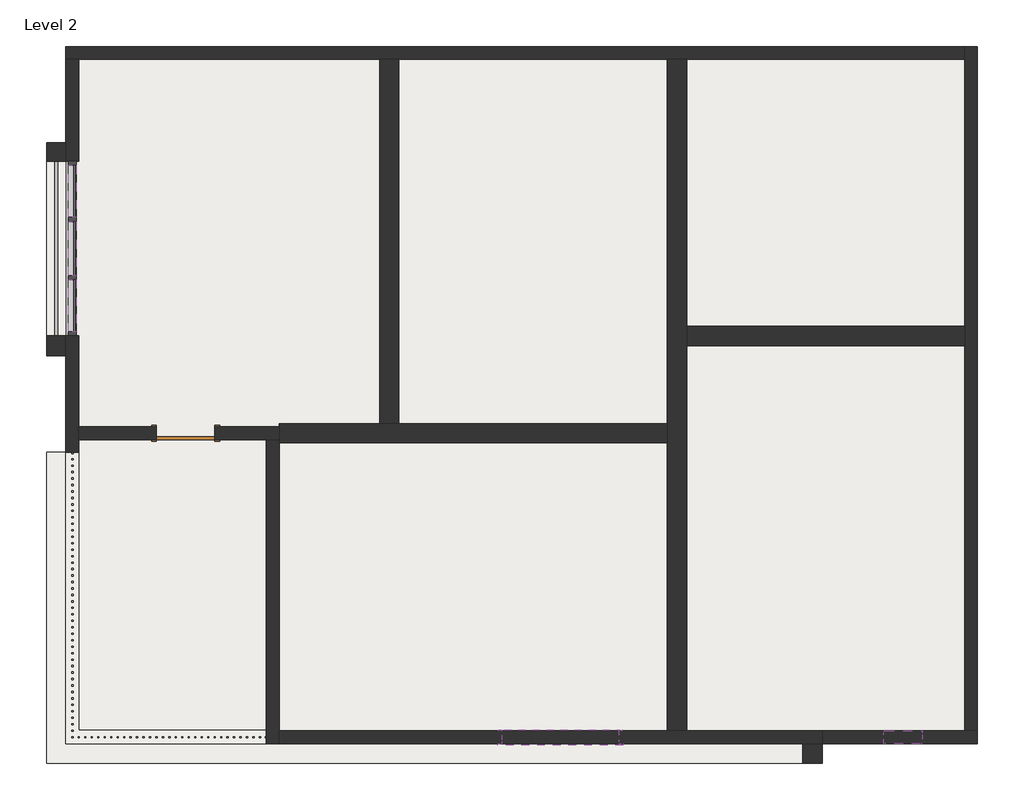
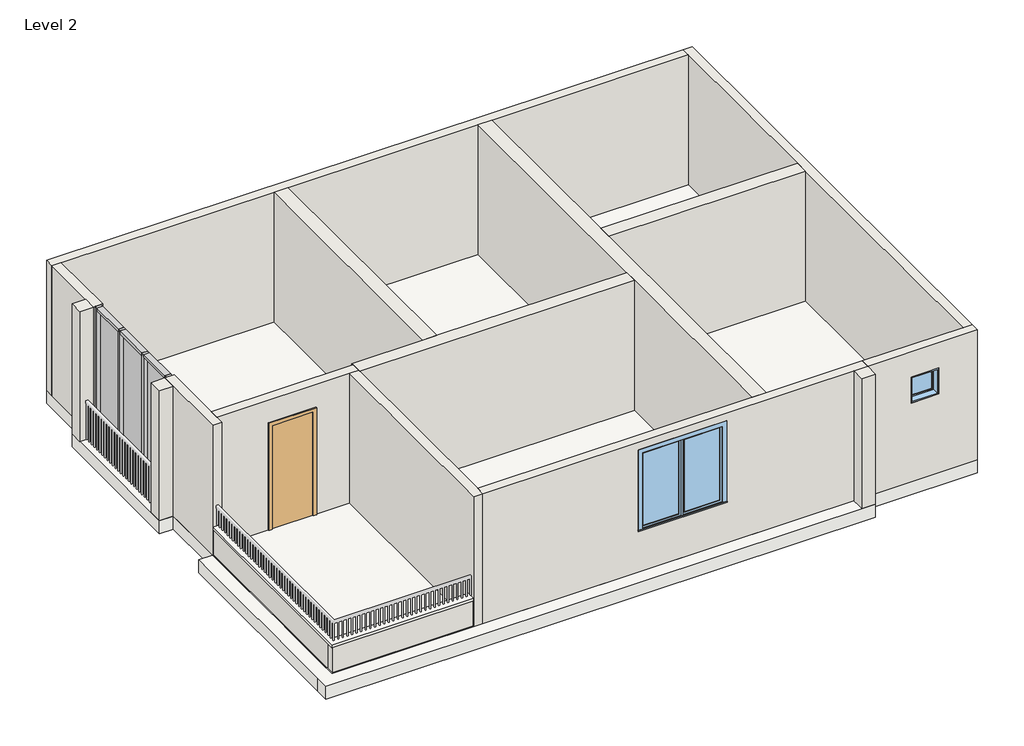
# One storey, part 1 of 2: 17 walls, 10 members, 3 plates, 3 slabs, 2 windows, 1 door.
"""IFC4 building model written with IfcOpenShell, lengths in millimetres."""

from ifc_helpers import new_model, si_unit, frame, origin, place, context, project, spatial, polyline, outline, extrude, faceted_brep, transform, mapped, element, save
from components import door_f936a269, member_eaba9652, member_3f395ae9, member_c17f1be2, member_d2e7e466, system_panel_glazed_52d31088, system_panel_glazed_f0722de2, window_97c6202a, window_6846e476

model = new_model("IFC4")

# Units and contexts
model_context = context("Model", 3, world=origin())
ifc_project = project(units=[si_unit("LENGTHUNIT", "METRE", prefix="MILLI")], contexts=[model_context])

# Site, building, storey
site = spatial("IfcSite", under=ifc_project)
building = spatial("IfcBuilding", under=site)
storey = spatial("IfcBuildingStorey", under=building, Name="Level 2", Elevation=3048.0)

# Door
placement = place(None, origin())
door_shape = door_f936a269(model_context)
element("IfcDoor", 1, ObjectType="Single-Flush : 36\" x 96\"", at=placement, inside=storey, context=model_context, shape_type="MappedRepresentation", body=[
    mapped(door_shape, transform((-16449.2169582, -4610.4617616, 3352.8), x_axis=(-1.0, 0.0, 0.0), y_axis=(0.0, -1.0, 0.0), z_axis=(0.0, 0.0, 1.0))),
])

# Members
member_shape = member_eaba9652(model_context)
element("IfcMember", 2, ObjectType="Rectangular Mullion : 2.5\" x 5\" rectangular", at=placement, inside=storey, context=model_context, shape_type="MappedRepresentation", body=[
    mapped(member_shape, transform((-18227.2169582, -1251.3117616, 3352.8), x_axis=(0.0, -1.0, 0.0), y_axis=(-1.0, 0.0, 0.0), z_axis=(0.0, 0.0, -1.0))),
])
element("IfcMember", 3, ObjectType="Rectangular Mullion : 2.5\" x 5\" rectangular", at=placement, inside=storey, context=model_context, shape_type="MappedRepresentation", body=[
    mapped(member_shape, transform((-18227.2169582, -2165.7117616, 3352.8), x_axis=(0.0, -1.0, 0.0), y_axis=(-1.0, 0.0, 0.0), z_axis=(0.0, 0.0, -1.0))),
])
member_2_shape = member_3f395ae9(model_context)
element("IfcMember", 4, ObjectType="Rectangular Mullion : 2.5\" x 5\" rectangular", at=placement, inside=storey, context=model_context, shape_type="MappedRepresentation", body=[
    mapped(member_2_shape, transform((-18227.2169582, -3080.1117616, 3352.8), x_axis=(0.0, -1.0, 0.0), y_axis=(-1.0, 0.0, 0.0), z_axis=(0.0, 0.0, -1.0))),
])
element("IfcMember", 5, ObjectType="Rectangular Mullion : 2.5\" x 5\" rectangular", at=placement, inside=storey, context=model_context, shape_type="MappedRepresentation", body=[
    mapped(member_2_shape, transform((-18227.2169582, -336.9117616, 6400.8), x_axis=(0.0, 1.0, 0.0), y_axis=(-1.0, 0.0, 0.0), z_axis=(0.0, 0.0, 1.0))),
])
member_3_shape = member_c17f1be2(model_context)
element("IfcMember", 6, ObjectType="Rectangular Mullion : 2.5\" x 5\" rectangular", at=placement, inside=storey, context=model_context, shape_type="MappedRepresentation", body=[
    mapped(member_3_shape, transform((-18227.2169582, -3016.6117616, 6400.8), x_axis=(0.0, 0.0, 1.0), y_axis=(-1.0, 0.0, 0.0), z_axis=(0.0, -1.0, 0.0))),
])
element("IfcMember", 7, ObjectType="Rectangular Mullion : 2.5\" x 5\" rectangular", at=placement, inside=storey, context=model_context, shape_type="MappedRepresentation", body=[
    mapped(member_3_shape, transform((-18227.2169582, -1219.5617616, 6400.8), x_axis=(0.0, 0.0, 1.0), y_axis=(-1.0, 0.0, 0.0), z_axis=(0.0, -1.0, 0.0))),
])
element("IfcMember", 8, ObjectType="Rectangular Mullion : 2.5\" x 5\" rectangular", at=placement, inside=storey, context=model_context, shape_type="MappedRepresentation", body=[
    mapped(member_3_shape, transform((-18227.2169582, -400.4117616, 3352.8), x_axis=(0.0, 0.0, -1.0), y_axis=(-1.0, 0.0, 0.0), z_axis=(0.0, 1.0, 0.0))),
])
element("IfcMember", 9, ObjectType="Rectangular Mullion : 2.5\" x 5\" rectangular", at=placement, inside=storey, context=model_context, shape_type="MappedRepresentation", body=[
    mapped(member_3_shape, transform((-18227.2169582, -2197.4617616, 3352.8), x_axis=(0.0, 0.0, -1.0), y_axis=(-1.0, 0.0, 0.0), z_axis=(0.0, 1.0, 0.0))),
])
member_4_shape = member_d2e7e466(model_context)
element("IfcMember", 10, ObjectType="Rectangular Mullion : 2.5\" x 5\" rectangular", at=placement, inside=storey, context=model_context, shape_type="MappedRepresentation", body=[
    mapped(member_4_shape, transform((-18227.2169582, -1283.0617616, 3352.8), x_axis=(0.0, 0.0, -1.0), y_axis=(-1.0, 0.0, 0.0), z_axis=(0.0, 1.0, 0.0))),
])
element("IfcMember", 11, ObjectType="Rectangular Mullion : 2.5\" x 5\" rectangular", at=placement, inside=storey, context=model_context, shape_type="MappedRepresentation", body=[
    mapped(member_4_shape, transform((-18227.2169582, -2133.9617616, 6400.8), x_axis=(0.0, 0.0, 1.0), y_axis=(-1.0, 0.0, 0.0), z_axis=(0.0, -1.0, 0.0))),
])

# Plates
system_panel_glazed_shape = system_panel_glazed_52d31088(model_context)
element("IfcPlate", 12, ObjectType="System Panel : Glazed", at=placement, inside=storey, context=model_context, shape_type="MappedRepresentation", body=[
    mapped(system_panel_glazed_shape, transform((-18227.2169582, -809.9867616, 3416.3), x_axis=(0.0, -1.0, 0.0), y_axis=(1.0, 0.0, 0.0), z_axis=(0.0, 0.0, 1.0))),
])
element("IfcPlate", 13, ObjectType="System Panel : Glazed", at=placement, inside=storey, context=model_context, shape_type="MappedRepresentation", body=[
    mapped(system_panel_glazed_shape, transform((-18227.2169582, -2607.0367616, 3416.3), x_axis=(0.0, -1.0, 0.0), y_axis=(1.0, 0.0, 0.0), z_axis=(0.0, 0.0, 1.0))),
])
system_panel_glazed_2_shape = system_panel_glazed_f0722de2(model_context)
element("IfcPlate", 14, ObjectType="System Panel : Glazed", at=placement, inside=storey, context=model_context, shape_type="MappedRepresentation", body=[
    mapped(system_panel_glazed_2_shape, transform((-18227.2169582, -1708.5117616, 3416.3), x_axis=(0.0, -1.0, 0.0), y_axis=(1.0, 0.0, 0.0), z_axis=(0.0, 0.0, 1.0))),
])

# Slabs
element("IfcSlab", 15, ObjectType="Generic - 12\"", at=placement, inside=storey, context=model_context, shape_type="SweptSolid", body=[
    extrude(outline(polyline([(-18633.6169582, -41.6299243), (-18328.8169582, -41.6299243), (-18328.8169582, -3394.4299243), (-18633.6169582, -3394.4299243), (-18633.6169582, -41.6299243)])), frame((0.0, 0.0, 3048.0), z_axis=(0.0, 0.0, 1.0), x_axis=(1.0, 0.0, 0.0)), (0.0, 0.0, 1.0), 304.8),
    extrude(outline(polyline([(-18633.6169582, -4908.9117616), (-18328.8169582, -4908.9117616), (-18328.8169582, -9487.2617616), (-6444.7919582, -9487.2617616), (-6444.7919582, -9792.0617616), (-18633.6169582, -9792.0617616), (-18633.6169582, -9487.2617616), (-18633.6169582, -4908.9117616)])), frame((0.0, 0.0, 3048.0), z_axis=(0.0, 0.0, 1.0), x_axis=(1.0, 0.0, 0.0)), (0.0, 0.0, 1.0), 304.8),
])
element("IfcSlab", 16, ObjectType="Generic - 12\" 2", at=placement, inside=storey, context=model_context, shape_type="SweptSolid", body=[
    extrude(outline(polyline([(-4006.3919582, 1466.4882384), (-4006.3919582, -9487.2617616), (-18328.8169582, -9487.2617616), (-18328.8169582, 1466.4882384), (-4006.3919582, 1466.4882384)])), frame((0.0, 0.0, 3048.0), z_axis=(0.0, 0.0, 1.0), x_axis=(1.0, 0.0, 0.0)), (0.0, 0.0, 1.0), 304.8),
])
element("IfcSlab", 17, ObjectType="Generic - 2\"", at=placement, inside=storey, context=model_context, shape_type="SweptSolid", body=[
    extrude(outline(polyline([(-15179.2169582, -9487.2617616), (-18328.8169582, -9487.2617616), (-18328.8169582, -4908.9117616), (-18125.6169582, -4908.9117616), (-18125.6169582, -9277.7117616), (-15179.2169582, -9277.7117616), (-15179.2169582, -9309.4617616), (-15179.2169582, -9487.2617616)])), frame((0.0, 0.0, 3962.4), z_axis=(0.0, 0.0, 1.0), x_axis=(1.0, 0.0, 0.0)), (0.0, 0.0, 1.0), 50.8),
])

# Walls
element("IfcWall", 18, ObjectType="Generic - 12\" white", at=placement, inside=storey, context=model_context, shape_type="SweptSolid", body=[
    extrude(outline(polyline([(-18633.6169582, -336.9117616), (-18633.6169582, -41.6299243), (-18328.8169582, -41.6299243), (-18328.8169582, -336.9117616), (-18633.6169582, -336.9117616)])), frame((0.0, 0.0, 3352.8), z_axis=(0.0, 0.0, 1.0), x_axis=(1.0, 0.0, 0.0)), (0.0, 0.0, 1.0), 3048.0),
])
element("IfcWall", 19, ObjectType="Generic - 12\" white", at=placement, inside=storey, context=model_context, shape_type="SweptSolid", body=[
    extrude(outline(polyline([(-18328.8169582, -3080.1117616), (-18328.8169582, -3394.4299243), (-18633.6169582, -3394.4299243), (-18633.6169582, -3080.1117616), (-18328.8169582, -3080.1117616)])), frame((0.0, 0.0, 3352.8), z_axis=(0.0, 0.0, 1.0), x_axis=(1.0, 0.0, 0.0)), (0.0, 0.0, 1.0), 3048.0),
])
element("IfcWall", 20, ObjectType="Generic - 12\" white", at=placement, inside=storey, context=model_context, shape_type="SweptSolid", body=[
    extrude(outline(polyline([(-6749.5919582, -9487.2617616), (-6444.7919582, -9487.2617616), (-6444.7919582, -9792.0617616), (-6749.5919582, -9792.0617616), (-6749.5919582, -9487.2617616)])), frame((0.0, 0.0, 3352.8), z_axis=(0.0, 0.0, 1.0), x_axis=(1.0, 0.0, 0.0)), (0.0, 0.0, 1.0), 3048.0),
])
element("IfcWall", 21, ObjectType="Generic - 12\" white", at=placement, inside=storey, context=model_context, shape_type="Brep", body=[
    faceted_brep([(-8575.2169582, -9284.0617616, 3352.8), (-8575.2169582, -3232.5117616, 3352.8), (-8575.2169582, -2927.7117616, 3352.8), (-8575.2169582, 1263.2882384, 3352.8), (-8575.2169582, 1263.2882384, 6400.8), (-8575.2169582, -2927.7117616, 6400.8), (-8575.2169582, -3232.5117616, 6400.8), (-8575.2169582, -9284.0617616, 6400.8), (-8880.0169582, -9284.0617616, 3352.8), (-8880.0169582, -9284.0617616, 6400.8), (-8880.0169582, -4762.8617616, 6400.8), (-8880.0169582, -4458.0617616, 6400.8), (-8880.0169582, 1263.2882384, 6400.8), (-8880.0169582, 1263.2882384, 3352.8), (-8880.0169582, -4458.0617616, 3352.8), (-8880.0169582, -4762.8617616, 3352.8)], [[[0, 1, 2, 3, 4, 5, 6, 7]], [[8, 9, 10, 11, 12, 13, 14, 15]], [[3, 2, 1, 0, 8, 15, 14, 13]], [[7, 6, 5, 4, 12, 11, 10, 9]], [[4, 3, 13, 12]], [[0, 7, 9, 8]]]),
])
element("IfcWall", 22, ObjectType="Generic - 12\" white", at=placement, inside=storey, context=model_context, shape_type="Brep", body=[
    faceted_brep([(-14976.0169582, -4762.8617616, 3352.8), (-8880.0169582, -4762.8617616, 3352.8), (-8880.0169582, -4762.8617616, 6400.8), (-14976.0169582, -4762.8617616, 6400.8), (-14976.0169582, -4458.0617616, 3352.8), (-14976.0169582, -4458.0617616, 6400.8), (-13401.2169582, -4458.0617616, 6400.8), (-13096.4169582, -4458.0617616, 6400.8), (-8880.0169582, -4458.0617616, 6400.8), (-8880.0169582, -4458.0617616, 3352.8), (-13096.4169582, -4458.0617616, 3352.8), (-13401.2169582, -4458.0617616, 3352.8), (-14976.0169582, -4712.0617616, 3352.8), (-14976.0169582, -4508.8617616, 3352.8), (-14976.0169582, -4508.8617616, 6400.8), (-14976.0169582, -4712.0617616, 6400.8)], [[[0, 1, 2, 3]], [[4, 5, 6, 7, 8, 9, 10, 11]], [[1, 0, 12, 13, 4, 11, 10, 9]], [[3, 2, 8, 7, 6, 5, 14, 15]], [[0, 3, 15, 14, 5, 4, 13, 12]], [[2, 1, 9, 8]]]),
])
element("IfcWall", 23, ObjectType="Generic - 12\" white", at=placement, inside=storey, context=model_context, shape_type="SweptSolid", body=[
    extrude(outline(polyline([(-13096.4169582, 1263.2882384), (-13096.4169582, -4458.0617616), (-13401.2169582, -4458.0617616), (-13401.2169582, 1263.2882384), (-13096.4169582, 1263.2882384)])), frame((0.0, 0.0, 3352.8), z_axis=(0.0, 0.0, 1.0), x_axis=(1.0, 0.0, 0.0)), (0.0, 0.0, 1.0), 3048.0),
])
element("IfcWall", 24, ObjectType="Generic - 12\" white", at=placement, inside=storey, context=model_context, shape_type="SweptSolid", body=[
    extrude(outline(polyline([(-4209.5919582, -3232.5117616), (-8575.2169582, -3232.5117616), (-8575.2169582, -2927.7117616), (-4209.5919582, -2927.7117616), (-4209.5919582, -3232.5117616)])), frame((0.0, 0.0, 3352.8), z_axis=(0.0, 0.0, 1.0), x_axis=(1.0, 0.0, 0.0)), (0.0, 0.0, 1.0), 3048.0),
])
element("IfcWall", 25, ObjectType="Generic - 6\"", at=placement, inside=storey, context=model_context, shape_type="Brep", body=[
    faceted_brep([(-15179.2169582, -9309.4617616, 3352.8), (-18151.0169582, -9309.4617616, 3352.8), (-18303.4169582, -9309.4617616, 3352.8), (-18303.4169582, -9309.4617616, 3962.4), (-18151.0169582, -9309.4617616, 3962.4), (-15179.2169582, -9309.4617616, 3962.4), (-15179.2169582, -9461.8617616, 3352.8), (-15179.2169582, -9461.8617616, 3962.4), (-18303.4169582, -9461.8617616, 3962.4), (-18303.4169582, -9461.8617616, 3352.8)], [[[0, 1, 2, 3, 4, 5]], [[6, 7, 8, 9]], [[2, 1, 0, 6, 9]], [[5, 4, 3, 8, 7]], [[0, 5, 7, 6]], [[3, 2, 9, 8]]]),
])
element("IfcWall", 26, ObjectType="Generic - 6\"", at=placement, inside=storey, context=model_context, shape_type="SweptSolid", body=[
    extrude(outline(polyline([(-18151.0169582, -4908.9117616), (-18151.0169582, -9309.4617616), (-18303.4169582, -9309.4617616), (-18303.4169582, -4908.9117616), (-18151.0169582, -4908.9117616)])), frame((0.0, 0.0, 3352.8), z_axis=(0.0, 0.0, 1.0), x_axis=(1.0, 0.0, 0.0)), (0.0, 0.0, 1.0), 609.6),
])
element("IfcWall", 27, ObjectType="Generic - 8\"", at=placement, inside=storey, context=model_context, shape_type="Brep", body=[
    faceted_brep([(-4006.3919582, -9284.0617616, 3352.8), (-4006.3919582, 1466.4882384, 3352.8), (-4006.3919582, 1466.4882384, 6400.8), (-4006.3919582, -9284.0617616, 6400.8), (-4209.5919582, -9284.0617616, 3352.8), (-4209.5919582, -9284.0617616, 6400.8), (-4209.5919582, -3232.5117616, 6400.8), (-4209.5919582, -2927.7117616, 6400.8), (-4209.5919582, 1263.2882384, 6400.8), (-4209.5919582, 1466.4882384, 6400.8), (-4209.5919582, 1466.4882384, 3352.8), (-4209.5919582, 1263.2882384, 3352.8), (-4209.5919582, -2927.7117616, 3352.8), (-4209.5919582, -3232.5117616, 3352.8)], [[[0, 1, 2, 3]], [[4, 5, 6, 7, 8, 9, 10, 11, 12, 13]], [[1, 0, 4, 13, 12, 11, 10]], [[3, 2, 9, 8, 7, 6, 5]], [[0, 3, 5, 4]], [[2, 1, 10, 9]]]),
])
element("IfcWall", 28, ObjectType="Generic - 8\"", at=placement, inside=storey, context=model_context, shape_type="Brep", body=[
    faceted_brep([(-4209.5919582, 1466.4882384, 3352.8), (-18328.8169582, 1466.4882384, 3352.8), (-18328.8169582, 1466.4882384, 6400.8), (-4209.5919582, 1466.4882384, 6400.8), (-4209.5919582, 1263.2882384, 3352.8), (-4209.5919582, 1263.2882384, 6400.8), (-8575.2169582, 1263.2882384, 6400.8), (-8880.0169582, 1263.2882384, 6400.8), (-13096.4169582, 1263.2882384, 6400.8), (-13401.2169582, 1263.2882384, 6400.8), (-18125.6169582, 1263.2882384, 6400.8), (-18328.8169582, 1263.2882384, 6400.8), (-18328.8169582, 1263.2882384, 3352.8), (-18125.6169582, 1263.2882384, 3352.8), (-13401.2169582, 1263.2882384, 3352.8), (-13096.4169582, 1263.2882384, 3352.8), (-8880.0169582, 1263.2882384, 3352.8), (-8575.2169582, 1263.2882384, 3352.8)], [[[0, 1, 2, 3]], [[4, 5, 6, 7, 8, 9, 10, 11, 12, 13, 14, 15, 16, 17]], [[1, 0, 4, 17, 16, 15, 14, 13, 12]], [[3, 2, 11, 10, 9, 8, 7, 6, 5]], [[0, 3, 5, 4]], [[2, 1, 12, 11]]]),
])
element("IfcWall", 29, ObjectType="Generic - 8\"", at=placement, inside=storey, context=model_context, shape_type="SweptSolid", body=[
    extrude(outline(polyline([(-18328.8169582, -336.9117616), (-18328.8169582, 1263.2882384), (-18125.6169582, 1263.2882384), (-18125.6169582, -336.9117616), (-18328.8169582, -336.9117616)])), frame((0.0, 0.0, 3352.8), z_axis=(0.0, 0.0, 1.0), x_axis=(1.0, 0.0, 0.0)), (0.0, 0.0, 1.0), 3048.0),
])
element("IfcWall", 30, ObjectType="Generic - 8\"", at=placement, inside=storey, context=model_context, shape_type="Brep", body=[
    faceted_brep([(-18328.8169582, -3080.1117616, 3352.8), (-18328.8169582, -4908.9117616, 3352.8), (-18328.8169582, -4908.9117616, 6400.8), (-18328.8169582, -3080.1117616, 6400.8), (-18125.6169582, -3080.1117616, 3352.8), (-18125.6169582, -3080.1117616, 6400.8), (-18125.6169582, -4508.8617616, 6400.8), (-18125.6169582, -4712.0617616, 6400.8), (-18125.6169582, -4908.9117616, 6400.8), (-18125.6169582, -4908.9117616, 3352.8), (-18125.6169582, -4712.0617616, 3352.8), (-18125.6169582, -4508.8617616, 3352.8), (-18151.0169582, -4908.9117616, 3352.8), (-18303.4169582, -4908.9117616, 3352.8)], [[[0, 1, 2, 3]], [[4, 5, 6, 7, 8, 9, 10, 11]], [[1, 0, 4, 11, 10, 9, 12, 13]], [[2, 1, 13, 12, 9, 8]], [[3, 2, 8, 7, 6, 5]], [[0, 3, 5, 4]]]),
])
element("IfcWall", 31, ObjectType="Generic - 8\" 2", at=placement, inside=storey, context=model_context, shape_type="Brep", body=[
    faceted_brep([(-4006.3919582, -9284.0617616, 3352.8), (-4209.5919582, -9284.0617616, 3352.8), (-6444.7919582, -9284.0617616, 3352.8), (-6444.7919582, -9284.0617616, 6400.8), (-4209.5919582, -9284.0617616, 6400.8), (-4006.3919582, -9284.0617616, 6400.8), (-4869.9919582, -9284.0617616, 5809.0087386), (-5479.5919582, -9284.0617616, 5809.0087386), (-5479.5919582, -9284.0617616, 5199.4087386), (-4869.9919582, -9284.0617616, 5199.4087386), (-4006.3919582, -9487.2617616, 3352.8), (-4006.3919582, -9487.2617616, 6400.8), (-6444.7919582, -9487.2617616, 6400.8), (-6444.7919582, -9487.2617616, 3352.8), (-4869.9919582, -9487.2617616, 5809.0087386), (-4869.9919582, -9487.2617616, 5199.4087386), (-5479.5919582, -9487.2617616, 5199.4087386), (-5479.5919582, -9487.2617616, 5809.0087386)], [[[0, 1, 2, 3, 4, 5], [6, 7, 8, 9]], [[10, 11, 12, 13], [14, 15, 16, 17]], [[2, 1, 0, 10, 13]], [[3, 2, 13, 12]], [[5, 4, 3, 12, 11]], [[0, 5, 11, 10]], [[15, 14, 6, 9]], [[16, 15, 9, 8]], [[17, 16, 8, 7]], [[14, 17, 7, 6]]]),
])
element("IfcWall", 32, ObjectType="Generic - 8\" 3", at=placement, inside=storey, context=model_context, shape_type="Brep", body=[
    faceted_brep([(-14976.0169582, -4712.0617616, 6400.8), (-15179.2169582, -4712.0617616, 6400.8), (-18125.6169582, -4712.0617616, 6400.8), (-18125.6169582, -4712.0617616, 3352.8), (-16906.4169582, -4712.0617616, 3352.8), (-16906.4169582, -4712.0617616, 5791.2), (-15992.0169582, -4712.0617616, 5791.2), (-15992.0169582, -4712.0617616, 3352.8), (-15179.2169582, -4712.0617616, 3352.8), (-14976.0169582, -4712.0617616, 3352.8), (-18125.6169582, -4508.8617616, 6400.8), (-14976.0169582, -4508.8617616, 6400.8), (-14976.0169582, -4508.8617616, 3352.8), (-15992.0169582, -4508.8617616, 3352.8), (-15992.0169582, -4508.8617616, 5791.2), (-16906.4169582, -4508.8617616, 5791.2), (-16906.4169582, -4508.8617616, 3352.8), (-18125.6169582, -4508.8617616, 3352.8)], [[[0, 1, 2, 3, 4, 5, 6, 7, 8, 9]], [[10, 11, 12, 13, 14, 15, 16, 17]], [[3, 17, 16, 4]], [[12, 9, 8, 7, 13]], [[2, 1, 0, 11, 10]], [[3, 2, 10, 17]], [[0, 9, 12, 11]], [[15, 5, 4, 16]], [[5, 15, 14, 6]], [[6, 14, 13, 7]]]),
])
element("IfcWall", 33, ObjectType="Generic - 8\" 3", at=placement, inside=storey, context=model_context, shape_type="Brep", body=[
    faceted_brep([(-15179.2169582, -4712.0617616, 3352.8), (-15179.2169582, -9309.4617616, 3352.8), (-15179.2169582, -9461.8617616, 3352.8), (-15179.2169582, -9487.2617616, 3352.8), (-15179.2169582, -9487.2617616, 6400.8), (-15179.2169582, -4712.0617616, 6400.8), (-14976.0169582, -4712.0617616, 3352.8), (-14976.0169582, -4712.0617616, 6400.8), (-14976.0169582, -4762.8617616, 6400.8), (-14976.0169582, -9284.0617616, 6400.8), (-14976.0169582, -9487.2617616, 6400.8), (-14976.0169582, -9487.2617616, 3352.8), (-14976.0169582, -9284.0617616, 3352.8), (-14976.0169582, -4762.8617616, 3352.8)], [[[0, 1, 2, 3, 4, 5]], [[6, 7, 8, 9, 10, 11, 12, 13]], [[3, 2, 1, 0, 6, 13, 12, 11]], [[5, 4, 10, 9, 8, 7]], [[0, 5, 7, 6]], [[3, 11, 10, 4]]]),
])
element("IfcWall", 34, ObjectType="Generic - 8\" 3", at=placement, inside=storey, context=model_context, shape_type="Brep", body=[
    faceted_brep([(-6444.7919582, -9284.0617616, 3352.8), (-8575.2169582, -9284.0617616, 3352.8), (-8880.0169582, -9284.0617616, 3352.8), (-14976.0169582, -9284.0617616, 3352.8), (-14976.0169582, -9284.0617616, 6400.8), (-8880.0169582, -9284.0617616, 6400.8), (-8575.2169582, -9284.0617616, 6400.8), (-6444.7919582, -9284.0617616, 6400.8), (-11470.8169582, -9284.0617616, 6151.0375963), (-11470.8169582, -9284.0617616, 4322.2375963), (-9642.0169582, -9284.0617616, 4322.2375963), (-9642.0169582, -9284.0617616, 6151.0375963), (-6444.7919582, -9487.2617616, 3352.8), (-6444.7919582, -9487.2617616, 6400.8), (-14976.0169582, -9487.2617616, 6400.8), (-14976.0169582, -9487.2617616, 3352.8), (-11470.8169582, -9487.2617616, 6151.0375963), (-9642.0169582, -9487.2617616, 6151.0375963), (-9642.0169582, -9487.2617616, 4322.2375963), (-11470.8169582, -9487.2617616, 4322.2375963)], [[[0, 1, 2, 3, 4, 5, 6, 7], [8, 9, 10, 11]], [[12, 13, 14, 15], [16, 17, 18, 19]], [[3, 2, 1, 0, 12, 15]], [[7, 6, 5, 4, 14, 13]], [[0, 7, 13, 12]], [[3, 15, 14, 4]], [[9, 8, 16, 19]], [[10, 9, 19, 18]], [[11, 10, 18, 17]], [[8, 11, 17, 16]]]),
])

# Windows
window_shape = window_97c6202a(model_context)
element("IfcWindow", 35, ObjectType="Casement Dbl with Trim.0001 : 72\" x 72\"", at=placement, inside=storey, context=model_context, shape_type="MappedRepresentation", body=[
    mapped(window_shape, transform((-10556.4169582, -9366.6117616, 3407.8375963), x_axis=(-1.0, 0.0, 0.0), y_axis=(0.0, -1.0, 0.0), z_axis=(0.0, 0.0, 1.0))),
])
window_2_shape = window_6846e476(model_context)
element("IfcWindow", 36, ObjectType="Fixed : 24\" x 24\"", at=placement, inside=storey, context=model_context, shape_type="MappedRepresentation", body=[
    mapped(window_2_shape, transform((-5136.6919582, -9385.6617616, 4285.0087386), x_axis=(1.0, 0.0, 0.0), y_axis=(0.0, 1.0, 0.0), z_axis=(0.0, 0.0, 1.0))),
])

save(model, "model.ifc")

# Revit data of these elements
# Type "Single-Flush : 36\" x 96\""
#   Type Mark = "1"
#   Construction Type Id = "MDOOR"
#   Assembly Code = "C1020"
#   Analytic Construction = "Metal"
#   Thickness = 0' - 2"
#   Heat Transfer Coefficient (U) = 0.651978 BTU/(h·ft²·°F)
#   Height = 8' - 0"
#   Trim Projection Ext = 0' - 1"
#   Trim Projection Int = 0' - 1"
#   Trim Width = 0' - 3"
#   Width = 3' - 0"
#   Define Thermal Properties by = 1
#   Door Material = Glass, Clear Glazing
#   Frame Material = Iron, Ductile
#   Visual Light Transmittance = 0
#   Solar Heat Gain Coefficient = 0
#   Function = (empty or 0)
#   Wall Closure = (empty or 0)
# Type "Rectangular Mullion : 2.5\" x 5\" rectangular"
#   built-in parameter 1007304 = 0.416667 (stored number, unit not read)
#   built-in parameter 1007301 = 0.104167 (stored number, unit not read)
#   built-in parameter 1007300 = 0.104167 (stored number, unit not read)
# Type "System Panel : Glazed"
#   Construction Type Id = "GSP4R"
#   Analytic Construction = "1/8 in Pilkington single glazing"
#   Visual Light Transmittance = 0.9
#   Solar Heat Gain Coefficient = 0.86
#   Heat Transfer Coefficient (U) = 1.18115 BTU/(h·ft²·°F)
# Type "Generic - 12\""
#   Assembly Code = "B1010"
#   Function = 0
#   Layers, outside or top first: 1' - 0" "Parking Stripe" (function 1)
# Type "Generic - 12\" 2"
#   Assembly Code = "B1010"
#   Function = 0
#   Layers, outside or top first: 1' - 0" "Parking Stripe" (function 1)
# Type "Generic - 2\""
#   Assembly Code = "B1010"
#   Function = 0
#   Layers, outside or top first: 0' - 2" "Parking Stripe" (function 1)
# Type "Generic - 12\" white"
#   Assembly Code = "B2010"
#   Layers, outside or top first: 1' - 0" "Parking Stripe" (function 1)
# Type "Generic - 6\""
#   Assembly Code = "B2010"
#   Layers, outside or top first: 0' - 6" "Concrete Masonry Units" (function 1)
# Type "Generic - 8\""
#   Assembly Code = "B2010"
#   Layers, outside or top first: 0' - 8" "Door - Frame" (function 1)
# Type "Generic - 8\" 2"
#   Assembly Code = "B2010"
#   Layers, outside or top first: 0' - 8" "Door - Frame" (function 1)
# Type "Generic - 8\" 3"
#   Assembly Code = "B2010"
#   Layers, outside or top first: 0' - 8" "EIFS, Exterior Insulation" (function 1)
# Type "Casement Dbl with Trim.0001 : 72\" x 72\""
#   Type Mark = "10"
#   Construction Type Id = "GSP4R"
#   Assembly Code = "B2020100"
#   Analytic Construction = "1/8 in Pilkington single glazing"
#   Visual Light Transmittance = 0.9
#   Solar Heat Gain Coefficient = 0.78
#   Heat Transfer Coefficient (U) = 0.6496 BTU/(h·ft²·°F)
#   Height = 6' - 0"
#   Default Sill Height = 3' - 0"
#   Trim Projection - Ext. = 0' - 0 1/2"
#   Trim Projection - Int. = 0' - 0 3/4"
#   Trim Width - Exterior = 0' - 3 1/2"
#   Trim Width - Interior = 0' - 3 1/2"
#   Width = 6' - 0"
#   Window Inset = 0' - 0 3/4"
#   Define Thermal Properties by = 1
#   Glass Pane Material = Glass
#   Sash Material = Iron, Ductile
#   Trim Exterior Material = Iron, Ductile
#   Trim Interior Material = Iron, Ductile
#   Wall Closure = (empty or 0)
# Type "Fixed : 24\" x 24\""
#   Type Mark = "3"
#   Construction Type Id = "GSP4R"
#   Assembly Code = "B2020100"
#   Analytic Construction = "1/8 in Pilkington single glazing"
#   Visual Light Transmittance = 0.9
#   Solar Heat Gain Coefficient = 0.78
#   Heat Transfer Coefficient (U) = 0.6496 BTU/(h·ft²·°F)
#   Height = 2' - 0"
#   Default Sill Height = 3' - 0"
#   Width = 2' - 0"
#   Window Inset = 0' - 0 3/4"
#   Define Thermal Properties by = 1
#   Glass Pane Material = Glass
#   Sash Material = Iron, Ductile
#   Wall Closure = (empty or 0)
# Element 1 (IfcDoor, "Single-Flush : 36\" x 96\"")
#   Phase Created = New Construction
#   Materials on its faces: "Iron, Ductile", "Glass, Clear Glazing"
# Elements 2, 3, 4, 5, 6, 7, 8, 9, 10, 11 (IfcMember, "Rectangular Mullion : 2.5\" x 5\" rectangular")
#   Phase Created = New Construction
#   Materials on its faces: "Iron, Ductile"
# Elements 12, 13, 14 (IfcPlate, "System Panel : Glazed")
#   Phase Created = New Construction
#   Materials on its faces: "Glass"
# Element 15 (IfcSlab, "Generic - 12\"")
#   built-in parameter 1001955 = 3.14159 (stored number, unit not read)
#   Height Offset From Level = 1' - 0"
#   Phase Created = New Construction
#   Materials on its faces: "Parking Stripe"
# Element 16 (IfcSlab, "Generic - 12\" 2")
#   Height Offset From Level = 1' - 0"
#   Phase Created = New Construction
#   Materials on its faces: "Parking Stripe"
# Element 17 (IfcSlab, "Generic - 2\"")
#   built-in parameter 1001955 = -1.5708 (stored number, unit not read)
#   Height Offset From Level = 3' - 2"
#   Phase Created = New Construction
#   Materials on its faces: "Parking Stripe"
# Elements 18, 19, 20, 21, 22, 23, 24 (IfcWall, "Generic - 12\" white")
#   built-in parameter 1001111 = 1' - 0"
#   Top Offset = 0' - 0"
#   Base Offset = 1' - 0"
#   Unconnected Height = 10' - 0"
#   wall height = 10' - 0"
#   Phase Created = New Construction
#   Base Constraint = Level 2
#   Materials on its faces: "Parking Stripe"
# Elements 25, 26 (IfcWall, "Generic - 6\"")
#   built-in parameter 1001111 = 1' - 0"
#   Top Offset = 0' - 0"
#   Base Offset = 1' - 0"
#   Unconnected Height = 2' - 0"
#   wall height = 2' - 0"
#   Phase Created = New Construction
#   Base Constraint = Level 2
#   Materials on its faces: "Concrete Masonry Units"
# Elements 27, 28, 29, 30 (IfcWall, "Generic - 8\"")
#   built-in parameter 1001111 = 1' - 0"
#   Top Offset = 0' - 0"
#   Base Offset = 1' - 0"
#   Unconnected Height = 10' - 0"
#   wall height = 10' - 0"
#   Phase Created = New Construction
#   Base Constraint = Level 2
#   Materials on its faces: "Door - Frame"
# Element 31 (IfcWall, "Generic - 8\" 2")
#   built-in parameter 1001111 = 1' - 0"
#   Top Offset = 0' - 0"
#   Base Offset = 1' - 0"
#   Unconnected Height = 10' - 0"
#   wall height = 10' - 0"
#   Phase Created = New Construction
#   Base Constraint = Level 2
#   Materials on its faces: "Door - Frame"
# Elements 32, 33, 34 (IfcWall, "Generic - 8\" 3")
#   built-in parameter 1001111 = 1' - 0"
#   Top Offset = 0' - 0"
#   Base Offset = 1' - 0"
#   Unconnected Height = 10' - 0"
#   wall height = 10' - 0"
#   Phase Created = New Construction
#   Base Constraint = Level 2
#   Materials on its faces: "EIFS, Exterior Insulation"
# Element 35 (IfcWindow, "Casement Dbl with Trim.0001 : 72\" x 72\"")
#   Mark = "2"
#   Phase Created = New Construction
#   Materials on its faces: "Iron, Ductile", "Glass"
# Element 36 (IfcWindow, "Fixed : 24\" x 24\"")
#   Mark = "1"
#   Phase Created = New Construction
#   Materials on its faces: "Iron, Ductile", "Glass"
# Materials
#   "Glass, Clear Glazing": class "Glass", colour RGB 0 128 192, transparency 0.75, Description = "Clear glazing", Cost = 0
#   "Iron, Ductile": class "Metal", colour RGB 0 0 0, transparency 0, Description = "Ductile cast iron", Cost = 0
#   "Parking Stripe": class "Paint", colour RGB 250 250 91, transparency 0, Cost = 0
#   "Concrete Masonry Units": class "Masonry", colour RGB 227 227 227, transparency 0, Description = "Concrete masonry units", Cost = 0
#   "Door - Frame": colour RGB 118 70 51, transparency 0, Cost = 0
#   "EIFS, Exterior Insulation": class "Generic", colour RGB 127 127 127, transparency 0, Description = "EIFS - Exterior Insulation", Cost = 0
#   "Glass": class "Glass", colour RGB 0 128 192, transparency 0.75, Description = "Soda Lime Glass", Cost = 0
